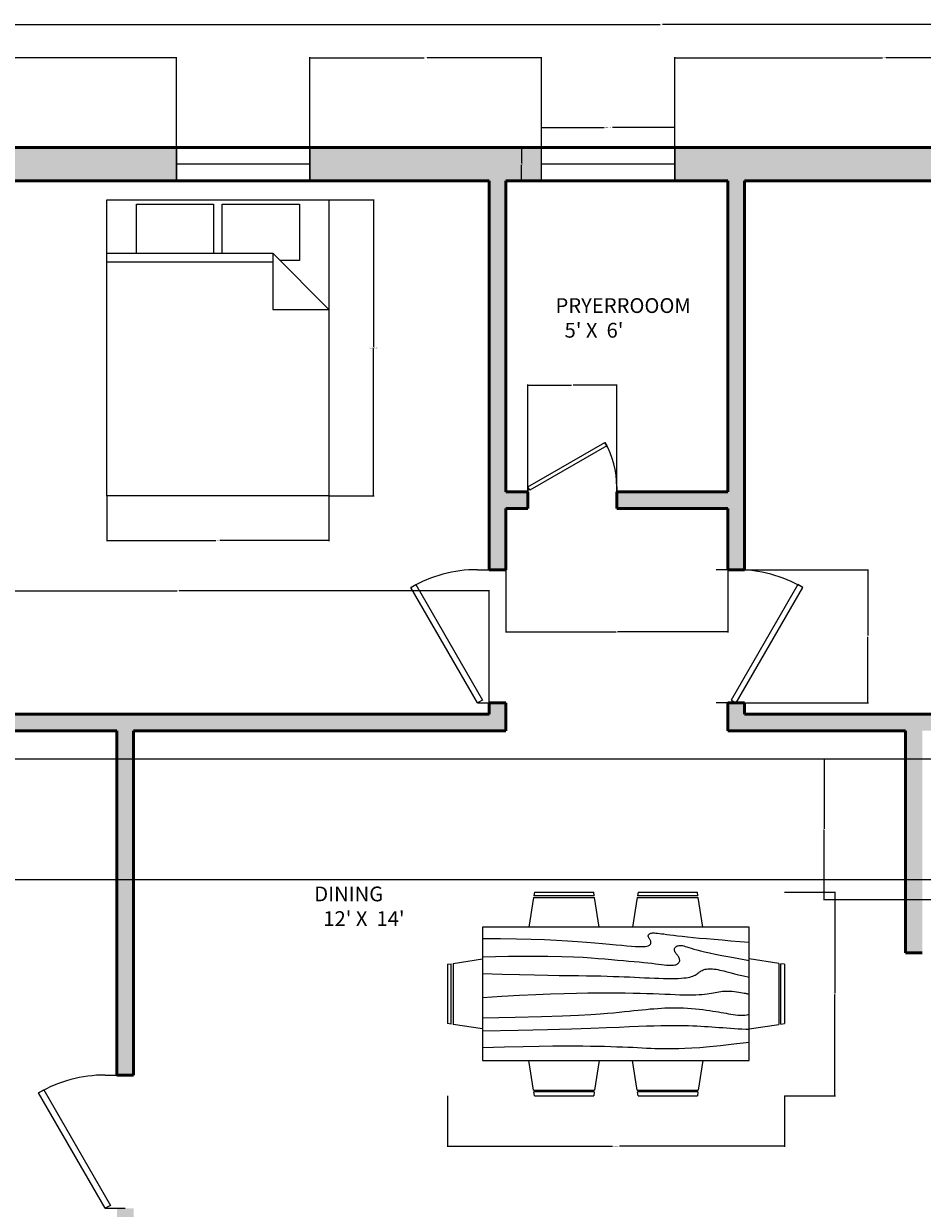
# Model space of a CAD drawing. Units: inches. Extents: x 4 to 671, y -79 to 570.
# Tile 4 of 7: x 165 to 408, y 250 to 570. Entities that reach past the tile are written whole.
import ezdxf

# ---------------------------------------------------------------- set-up
doc = ezdxf.new("R2010")
doc.units = ezdxf.units.IN
doc.header["$MEASUREMENT"] = 0
for name, color, linetype, lineweight in [('A-ANNO-DIMS', 2, 'Continuous', 18), ('A-AREA-IDEN', 7, 'Continuous', 18), ('A-WALL', 7, 'Continuous', 50), ('A-WALL-PATT', 251, 'Continuous', 13), ('doors', 40, 'Continuous', 25), ('furniture', 220, 'Continuous', 18), ('window', 30, 'Continuous', 25)]:
    doc.layers.add(name, color=color, linetype=linetype, lineweight=lineweight)
doc.styles.get("Standard").update_dxf_attribs({"font": 'arial.ttf'})
doc.dimstyles.get("Standard").update_dxf_attribs({"dimtxt": 0.18, "dimasz": 0.18, "dimexe": 0.18, "dimexo": 0.0625, "dimgap": 0.09, "dimtad": 0, "dimtih": 1, "dimtoh": 1, "dimdec": 4, "dimzin": 0, "dimdsep": 46, "dimtxsty": 'Standard', "dimcen": 0.09, "dimadec": 0, "dimazin": 0, "dimtfac": 1, "dimtdec": 4, "dimtofl": 0, "dimtmove": 0, "dimatfit": 3, "dimfxl": 1, "dimtolj": 1, "dimtzin": 0, "dimarcsym": 0})

# ---------------------------------------------------------------- blocks, each defined once
blk = doc.blocks.new('*U10')
for p, q in [((0, 0), (0, 6)), ((40, 0), (40, 6))]:
    blk.add_line(p, q)
blk.add_lwpolyline([(0, 0), (34.64, -20), (35.52, -18.48), (0.87, 1.52)], close=True)
blk.add_arc((0, 0), 40, 330, 0)
blk = doc.blocks.new('*U9')
for p, q in [((0, 0), (0, -6)), ((40, 0), (40, -6))]:
    blk.add_line(p, q)
blk.add_lwpolyline([(0, 0), (34.64, 20), (35.52, 18.48), (0.87, -1.52)], close=True)
blk.add_arc((0, 0), 40, 0, 30)
blk = doc.blocks.new('Bed - Queen')
for p, q in [((0, -80.00003), (0, 0)), ((0, 0), (59.99999, 0)), ((59.99999, 0), (59.99999, -80.00003)), ((7.99999, -1.2), (28.79998, -1.2)), ((7.99999, -14.4), (7.99999, -1.2)), ((28.79998, -1.2), (28.79998, -14.4)), ((31.19999, -1.2), (51.99999, -1.2)), ((31.19999, -14.4), (31.19999, -1.2)), ((51.99999, -1.2), (51.99999, -16.4)), ((0, -14.4), (44.8, -14.4)), ((59.99999, -29.6), (44.8, -14.4)), ((44.8, -14.4), (44.8, -29.6)), ((44.8, -16.8), (0, -16.8)), ((51.99999, -16.4), (46.79936, -16.4)), ((44.8, -29.6), (59.99999, -29.6)), ((59.99999, -80.00003), (0, -80.00003))]:
    blk.add_line(p, q)
blk = doc.blocks.new('Dining Set - 36 x 72 in.')
for p, q in [((-22.2343, 26.00059), (-23.4847, 17.99762)), ((-22.2304, 26), (-5.7608, 26)), ((-22, 27.5), (-22.1562, 26.50042)), ((-5.8416, 26.5), (-22.1534, 26.5)), ((-22, 27.5), (-6, 27.5)), ((-5.8437, 26.49966), (-6, 27.5)), ((-4.5152, 17.99762), (-5.7655, 25.99926)), ((5.7657, 26.00059), (4.5153, 17.99762)), ((5.7696, 26), (22.2392, 26)), ((6, 27.5), (5.8438, 26.50042)), ((22.1584, 26.5), (5.8466, 26.5)), ((6, 27.5), (22, 27.5)), ((22.1563, 26.49966), (22, 27.5)), ((23.4848, 17.99762), (22.2345, 25.99926)), ((36, 18), (-36, 18)), ((-36, 18), (-36, -18)), ((36, -18), (36, 18)), ((-45.5, 8), (-44.5004, 8.15617)), ((-45.5, 8), (-45.5, -8)), ((-44.5, -8.15843), (-44.5, 8.15338)), ((-44.0006, 8.23428), (-35.9976, 9.48474)), ((-44, 8.23041), (-44, -8.23915)), ((44.0006, 8.23428), (35.9976, 9.48474)), ((44, 8.23041), (44, -8.23915)), ((44.5, -8.15843), (44.5, 8.15338)), ((45.5, 8), (44.5005, 8.15617)), ((45.5, 8), (45.5, -8)), ((-44.4997, -8.15631), (-45.5, -8)), ((-35.9976, -9.48476), (-43.9993, -8.2345)), ((35.9976, -9.48476), (43.9993, -8.2345)), ((44.4997, -8.15631), (45.5, -8)), ((-36, -18), (36, -18)), ((-22.2343, -26.0006), (-23.4847, -17.99762)), ((-4.5152, -17.99762), (-5.7655, -25.99928)), ((5.7657, -26.0006), (4.5153, -17.99762)), ((23.4848, -17.99762), (22.2345, -25.99928)), ((-22.2304, -26), (-5.7608, -26)), ((-22, -27.5), (-22.1562, -26.50044)), ((-5.8416, -26.5), (-22.1534, -26.5)), ((-22, -27.5), (-6, -27.5)), ((-5.8437, -26.49967), (-6, -27.5)), ((5.7696, -26), (22.2392, -26)), ((6, -27.5), (5.8438, -26.50044)), ((22.1584, -26.5), (5.8466, -26.5)), ((6, -27.5), (22, -27.5)), ((22.1563, -26.49967), (22, -27.5))]:
    blk.add_line(p, q)
for points in [[(-36, 15), (-31.1772, 14.97754), (-26.8079, 14.91406), (-22.8538, 14.81543), (-19.276, 14.6875), (-16.0362, 14.53613), (-13.0957, 14.36718), (-10.4159, 14.18652), (-7.9583, 14), (-5.6904, 13.81315), (-3.6035, 13.63021), (-1.6954, 13.45508), (0.0365, 13.29166), (1.5945, 13.14388), (2.9811, 13.01562), (4.1988, 12.9108), (5.25, 12.83333), (6.1393, 12.78613), (6.8802, 12.76823), (7.4883, 12.77767), (7.9792, 12.8125), (8.3685, 12.87077), (8.6719, 12.95052), (8.9049, 13.0498), (9.0833, 13.16666), (9.2205, 13.29899), (9.3216, 13.44401), (9.3895, 13.59879), (9.4271, 13.76041), (9.4373, 13.92594), (9.4232, 14.09245), (9.3875, 14.257), (9.3333, 14.41666), (9.2638, 14.56917), (9.1836, 14.71484), (9.0975, 14.85465), (9.0104, 14.98958), (8.9272, 15.1206), (8.8529, 15.2487), (8.7922, 15.37483), (8.75, 15.5), (8.7305, 15.62467), (8.7344, 15.74739), (8.7617, 15.86621), (8.8125, 15.97916), (8.8867, 16.08431), (8.9844, 16.17968), (9.1055, 16.26334), (9.25, 16.33333), (9.4189, 16.38802), (9.6172, 16.42708), (9.8506, 16.45052), (10.125, 16.45833), (10.4463, 16.45052), (10.8203, 16.42708), (11.2529, 16.38802), (11.75, 16.33333), (12.3184, 16.26318), (12.9694, 16.17838), (13.7151, 16.07991), (14.5677, 15.96875), (15.5395, 15.84586), (16.6426, 15.71224), (17.8893, 15.56884), (19.2917, 15.41666), (20.859, 15.25667), (22.5879, 15.08984), (24.4721, 14.91715), (26.5052, 14.73958), (28.6809, 14.5581), (30.9929, 14.3737), (33.4347, 14.18733), (36, 14)], [(-36, 10), (-28.9766, 10.14274), (-23.1725, 10.20442), (-18.4241, 10.19775), (-14.5677, 10.13541), (-11.4399, 10.03011), (-8.877, 9.89453), (-6.7154, 9.74137), (-4.7917, 9.58333), (-2.9698, 9.43082), (-1.2246, 9.28515), (0.4415, 9.14534), (2.026, 9.01041), (3.5266, 8.87939), (4.9408, 8.7513), (6.266, 8.62516), (7.5, 8.5), (8.6411, 8.37549), (9.6914, 8.2539), (10.6538, 8.13818), (11.5312, 8.03125), (12.3267, 7.93603), (13.043, 7.85547), (13.6831, 7.79248), (14.25, 7.75), (14.7471, 7.7303), (15.1797, 7.73307), (15.5537, 7.75732), (15.875, 7.80208), (16.1494, 7.86637), (16.3828, 7.94922), (16.5811, 8.04964), (16.75, 8.16666), (16.8944, 8.29915), (17.0143, 8.44531), (17.1089, 8.60319), (17.1771, 8.77083), (17.218, 8.94629), (17.2305, 9.1276), (17.2137, 9.31282), (17.1667, 9.5), (17.0895, 9.6875), (16.987, 9.875), (16.8649, 10.0625), (16.7292, 10.25), (16.5856, 10.4375), (16.4401, 10.625), (16.2985, 10.8125), (16.1667, 11), (16.05, 11.18733), (15.9518, 11.3737), (15.8752, 11.5581), (15.8229, 11.73958), (15.798, 11.91715), (15.8034, 12.08984), (15.842, 12.25667), (15.9167, 12.41666), (16.0295, 12.56836), (16.1784, 12.70833), (16.3605, 12.83268), (16.5729, 12.9375), (16.8127, 13.01888), (17.0768, 13.07291), (17.3625, 13.0957), (17.6667, 13.08333), (17.9894, 13.03312), (18.3418, 12.94726), (18.7382, 12.82918), (19.1927, 12.68229), (19.7195, 12.51001), (20.3327, 12.31575), (21.0465, 12.10294), (21.875, 11.875), (22.8357, 11.63354), (23.959, 11.37304), (25.2786, 11.08618), (26.8282, 10.76562), (28.6414, 10.40405), (30.752, 9.99414), (33.1936, 9.52856), (36, 9)], [(-36, 5.5), (-30.7157, 5.3348), (-26.069, 5.20963), (-21.9946, 5.11767), (-18.4271, 5.05208), (-15.3009, 5.00602), (-12.5508, 4.97265), (-10.1112, 4.94515), (-7.9167, 4.91666), (-5.909, 4.88167), (-4.0586, 4.83984), (-2.3429, 4.79215), (-0.7396, 4.73958), (0.7739, 4.6831), (2.22, 4.6237), (3.6213, 4.56233), (5, 4.5), (6.373, 4.43782), (7.7344, 4.3776), (9.0723, 4.32129), (10.375, 4.27083), (11.6309, 4.22819), (12.8281, 4.19531), (13.9551, 4.17415), (15, 4.16666), (15.954, 4.17448), (16.819, 4.19791), (17.6001, 4.23698), (18.3021, 4.29166), (18.9299, 4.36198), (19.4883, 4.44791), (19.9823, 4.54948), (20.4167, 4.66666), (20.7969, 4.79899), (21.1302, 4.94401), (21.4245, 5.09879), (21.6875, 5.26041), (21.9271, 5.42594), (22.1511, 5.59245), (22.3672, 5.757), (22.5834, 5.91666), (22.8065, 6.06868), (23.0404, 6.21093), (23.2879, 6.34147), (23.5521, 6.45833), (23.8358, 6.55957), (24.142, 6.64323), (24.4735, 6.70735), (24.8334, 6.75), (25.2235, 6.76969), (25.642, 6.76692), (26.0858, 6.74267), (26.5521, 6.69791), (27.0379, 6.63362), (27.5404, 6.55078), (28.0565, 6.45036), (28.5834, 6.33333), (29.1242, 6.19987), (29.7071, 6.04687), (30.3661, 5.87044), (31.1354, 5.66666), (32.0493, 5.43164), (33.142, 5.16146), (34.4475, 4.85221), (36, 4.5)], [(-36, -1), (-30.7915, -0.6591), (-26.0195, -0.38216), (-21.6519, -0.16284), (-17.6563, 0.00521), (-14.0005, 0.12833), (-10.6523, 0.21289), (-7.5796, 0.26522), (-4.75, 0.29166), (-2.134, 0.29793), (0.2878, 0.28711), (2.5317, 0.26163), (4.6146, 0.22396), (6.5529, 0.17651), (8.3633, 0.12174), (10.0623, 0.06209), (11.6667, 0), (13.1899, -0.06201), (14.6341, -0.1211), (15.9982, -0.17432), (17.2813, -0.21875), (18.4823, -0.25147), (19.6003, -0.26953), (20.6343, -0.27002), (21.5834, -0.25), (22.4481, -0.20768), (23.2357, -0.14584), (23.9549, -0.06836), (24.6146, 0.02083), (25.2235, 0.11784), (25.7904, 0.21875), (26.3241, 0.31966), (26.8334, 0.41666), (27.3265, 0.50618), (27.8099, 0.58593), (28.2894, 0.65397), (28.7709, 0.70833), (29.2601, 0.74707), (29.763, 0.76823), (30.2855, 0.76985), (30.8334, 0.75), (31.4088, 0.70784), (31.9994, 0.64713), (32.589, 0.57275), (33.1615, 0.48958), (33.7008, 0.4025), (34.1908, 0.3164), (34.6153, 0.23616), (34.9584, 0.16666), (35.2099, 0.11165), (35.3848, 0.07031), (35.504, 0.04069), (35.5886, 0.02083), (35.6594, 0.00879), (35.7377, 0.0026), (35.8442, 0.00032), (36, 0)], [(-36, -6.5), (-27.1843, -6.31267), (-20.084, -6.1263), (-14.469, -5.9419), (-10.1094, -5.76042), (-6.7752, -5.58285), (-4.2363, -5.41016), (-2.2629, -5.24333), (-0.625, -5.08334), (0.8708, -4.93099), (2.2715, -4.78646), (3.5872, -4.64974), (4.8281, -4.52084), (6.0046, -4.39974), (7.127, -4.28646), (8.2053, -4.18099), (9.25, -4.08334), (10.2705, -3.99382), (11.2734, -3.91407), (12.2647, -3.84603), (13.25, -3.79167), (14.2354, -3.75293), (15.2266, -3.73177), (16.2295, -3.73015), (17.25, -3.75), (18.2912, -3.79248), (19.3451, -3.85547), (20.4009, -3.93604), (21.4479, -4.03125), (22.4754, -4.13819), (23.4727, -4.25391), (24.4289, -4.37549), (25.3334, -4.5), (26.1785, -4.62492), (26.9694, -4.74935), (27.7145, -4.87281), (28.4219, -4.99479), (29.1, -5.11483), (29.7572, -5.23242), (30.4016, -5.34709), (31.0417, -5.45834), (31.6837, -5.56437), (32.3262, -5.65821), (32.9658, -5.73153), (33.599, -5.77604), (34.2224, -5.78345), (34.8327, -5.74545), (35.4264, -5.65373), (36, -5.5)], [(-36, -10), (-26.4022, -9.81299), (-18.4675, -9.62891), (-11.9839, -9.45069), (-6.7396, -9.28125), (-2.5226, -9.12354), (0.8789, -8.98047), (3.6769, -8.85498), (6.0833, -8.75), (8.2767, -8.66765), (10.3021, -8.60677), (12.1712, -8.56543), (13.8958, -8.54167), (15.4876, -8.53353), (16.9583, -8.53907), (18.3197, -8.55632), (19.5834, -8.58334), (20.7616, -8.61841), (21.8685, -8.66081), (22.9188, -8.71004), (23.9271, -8.76563), (24.9081, -8.82707), (25.8763, -8.89388), (26.8465, -8.96558), (27.8334, -9.04167), (28.8474, -9.12118), (29.8828, -9.20117), (30.93, -9.27824), (31.9792, -9.34896), (33.0205, -9.40991), (34.0443, -9.45768), (35.0407, -9.48885), (36, -9.5)], [(-36, -14.5), (-30.0881, -14.33513), (-25.0332, -14.21224), (-20.7312, -14.12647), (-17.0781, -14.07292), (-13.97, -14.04671), (-11.3027, -14.04297), (-8.9724, -14.05681), (-6.875, -14.08334), (-4.9224, -14.11833), (-3.0905, -14.16016), (-1.3709, -14.20785), (0.2448, -14.26042), (1.7647, -14.3169), (3.1973, -14.3763), (4.5507, -14.43767), (5.8333, -14.5), (7.0554, -14.5621), (8.235, -14.62175), (9.3922, -14.67652), (10.5469, -14.72396), (11.7192, -14.76164), (12.929, -14.78711), (14.1965, -14.79794), (15.5417, -14.79167), (16.9933, -14.76424), (18.6152, -14.70508), (20.4804, -14.60197), (22.6615, -14.44271), (25.2312, -14.21509), (28.2624, -13.9069), (31.8277, -13.50594), (36, -13)]]:
    blk.add_lwpolyline(points)
blk = doc.blocks.new('WIN-36')
for p, q in [((0, 0), (0, 9)), ((0, 9), (36, 9)), ((36, 9), (36, 0)), ((36, 9), (36, 4.5)), ((36, 4.5), (0, 4.5)), ((36, 0), (0, 0))]:
    blk.add_line(p, q)
blk = doc.blocks.new('*D21')
at = {"layer": 'A-ANNO-DIMS', "color": 0, "lineweight": -2, "transparency": 16777216}
for p, q in [((305.11, 536.41), (305.11, 541.93)), ((305.29, 541.75), (321.99, 541.75)), ((340.93, 541.75), (324.23, 541.75)), ((341.11, 536.41), (341.11, 541.93))]:
    blk.add_line(p, q, dxfattribs=at)
at = {"layer": 'A-ANNO-DIMS', "color": 0, "transparency": 16777216}
for points in [[(305.29, 541.78), (305.29, 541.72), (305.11, 541.75)], [(340.93, 541.78), (340.93, 541.72), (341.11, 541.75)]]:
    blk.add_solid(points, dxfattribs=at)
at = {"layer": 'Defpoints', "color": 0, "transparency": 16777216}
for p in [(341.11, 541.75), (305.11, 536.35), (341.11, 536.35)]:
    blk.add_point(p, dxfattribs=at)
at = {"layer": 'A-ANNO-DIMS', "color": 0, "transparency": 16777216, "insert": (323.11, 541.75), "char_height": 0.18, "attachment_point": 5}
blk.add_mtext('\\A1;WINDOW 36 TYP.', dxfattribs=at)
blk = doc.blocks.new('*D22')
at = {"layer": 'A-ANNO-DIMS', "color": 0, "lineweight": -2, "transparency": 16777216}
for p, q in [((305.05, 536.35), (299.53, 536.35)), ((299.71, 536.17), (299.71, 532.03)), ((299.71, 527.53), (299.71, 531.67)), ((305.05, 527.35), (299.53, 527.35))]:
    blk.add_line(p, q, dxfattribs=at)
at = {"layer": 'A-ANNO-DIMS', "color": 0, "transparency": 16777216}
for points in [[(299.68, 536.17), (299.74, 536.17), (299.71, 536.35)], [(299.68, 527.53), (299.74, 527.53), (299.71, 527.35)]]:
    blk.add_solid(points, dxfattribs=at)
at = {"layer": 'Defpoints', "color": 0, "transparency": 16777216}
for p in [(299.71, 536.35), (305.11, 536.35), (305.11, 527.35)]:
    blk.add_point(p, dxfattribs=at)
at = {"layer": 'A-ANNO-DIMS', "color": 0, "transparency": 16777216, "insert": (299.71, 531.85), "char_height": 0.18, "attachment_point": 5}
blk.add_mtext('\\A1;9 TYP.', dxfattribs=at)
blk = doc.blocks.new('*D27')
at = {"layer": 'A-ANNO-DIMS', "color": 0, "lineweight": -2, "transparency": 16777216}
for p, q in [((247.76, 522.26), (259.87, 522.26)), ((259.69, 522.08), (259.69, 482.45)), ((259.69, 442.44), (259.69, 482.07)), ((247.76, 442.26), (259.87, 442.26))]:
    blk.add_line(p, q, dxfattribs=at)
at = {"layer": 'A-ANNO-DIMS', "color": 0, "transparency": 16777216}
for points in [[(259.66, 522.08), (259.72, 522.08), (259.69, 522.26)], [(259.66, 442.44), (259.72, 442.44), (259.69, 442.26)]]:
    blk.add_solid(points, dxfattribs=at)
at = {"layer": 'Defpoints', "color": 0, "transparency": 16777216}
for p in [(247.69, 522.26), (259.69, 522.26), (247.69, 442.26)]:
    blk.add_point(p, dxfattribs=at)
at = {"layer": 'A-ANNO-DIMS', "color": 0, "transparency": 16777216, "insert": (259.69, 482.26), "char_height": 0.18, "attachment_point": 5}
blk.add_mtext('\\A1;QUEEN BED 80 TYP.', dxfattribs=at)
blk = doc.blocks.new('*D28')
at = {"layer": 'A-ANNO-DIMS', "color": 0, "lineweight": -2, "transparency": 16777216}
for p, q in [((187.69, 442.2), (187.69, 430.08)), ((247.69, 442.2), (247.69, 430.08)), ((187.87, 430.26), (217.17, 430.26)), ((247.51, 430.26), (218.22, 430.26))]:
    blk.add_line(p, q, dxfattribs=at)
at = {"layer": 'A-ANNO-DIMS', "color": 0, "transparency": 16777216}
for points in [[(187.87, 430.29), (187.87, 430.23), (187.69, 430.26)], [(247.51, 430.29), (247.51, 430.23), (247.69, 430.26)]]:
    blk.add_solid(points, dxfattribs=at)
at = {"layer": 'Defpoints', "color": 0, "transparency": 16777216}
for p in [(187.69, 442.26), (247.69, 442.26), (247.69, 430.26)]:
    blk.add_point(p, dxfattribs=at)
at = {"layer": 'A-ANNO-DIMS', "color": 0, "transparency": 16777216, "insert": (217.69, 430.26), "char_height": 0.18, "attachment_point": 5}
blk.add_mtext('\\A1;60 TYP.', dxfattribs=at)
blk = doc.blocks.new('*D41')
at = {"layer": 'A-ANNO-DIMS', "color": 0, "lineweight": -2, "transparency": 16777216}
for p, q in [((279.69, 280.21), (279.69, 266.44)), ((370.69, 280.21), (370.69, 266.44)), ((279.87, 266.62), (324.24, 266.62)), ((370.51, 266.62), (326.15, 266.62))]:
    blk.add_line(p, q, dxfattribs=at)
at = {"layer": 'A-ANNO-DIMS', "color": 0, "transparency": 16777216}
for points in [[(279.87, 266.65), (279.87, 266.59), (279.69, 266.62)], [(370.51, 266.65), (370.51, 266.59), (370.69, 266.62)]]:
    blk.add_solid(points, dxfattribs=at)
at = {"layer": 'Defpoints', "color": 0, "transparency": 16777216}
for p in [(279.69, 280.27), (370.69, 280.27), (370.69, 266.62)]:
    blk.add_point(p, dxfattribs=at)
at = {"layer": 'A-ANNO-DIMS', "color": 0, "transparency": 16777216, "insert": (325.19, 266.62), "char_height": 0.18, "attachment_point": 5}
blk.add_mtext('\\A1;DINING SET 91', dxfattribs=at)
blk = doc.blocks.new('*D42')
at = {"layer": 'A-ANNO-DIMS', "color": 0, "lineweight": -2, "transparency": 16777216}
for p, q in [((370.76, 335.27), (384.52, 335.27)), ((384.34, 335.09), (384.34, 307.95)), ((384.34, 280.45), (384.34, 307.59)), ((370.76, 280.27), (384.52, 280.27))]:
    blk.add_line(p, q, dxfattribs=at)
at = {"layer": 'A-ANNO-DIMS', "color": 0, "transparency": 16777216}
for points in [[(384.31, 335.09), (384.37, 335.09), (384.34, 335.27)], [(384.31, 280.45), (384.37, 280.45), (384.34, 280.27)]]:
    blk.add_solid(points, dxfattribs=at)
at = {"layer": 'Defpoints', "color": 0, "transparency": 16777216}
for p in [(370.69, 335.27), (384.34, 335.27), (370.69, 280.27)]:
    blk.add_point(p, dxfattribs=at)
at = {"layer": 'A-ANNO-DIMS', "color": 0, "transparency": 16777216, "insert": (384.34, 307.77), "char_height": 0.18, "attachment_point": 5}
blk.add_mtext('\\A1;55', dxfattribs=at)
blk = doc.blocks.new('*D49')
at = {"layer": 'A-ANNO-DIMS', "color": 0, "lineweight": -2, "transparency": 16777216}
for p, q in [((37.44, 536.41), (37.44, 569.83)), ((37.62, 569.65), (337.15, 569.65)), ((637.26, 569.65), (337.73, 569.65)), ((637.44, 536.41), (637.44, 569.83))]:
    blk.add_line(p, q, dxfattribs=at)
at = {"layer": 'A-ANNO-DIMS', "color": 0, "transparency": 16777216}
for points in [[(37.62, 569.68), (37.62, 569.62), (37.44, 569.65)], [(637.26, 569.68), (637.26, 569.62), (637.44, 569.65)]]:
    blk.add_solid(points, dxfattribs=at)
at = {"layer": 'Defpoints', "color": 0, "transparency": 16777216}
for p in [(637.44, 569.65), (37.44, 536.35), (637.44, 536.35)]:
    blk.add_point(p, dxfattribs=at)
at = {"layer": 'A-ANNO-DIMS', "color": 0, "transparency": 16777216, "insert": (337.44, 569.65), "char_height": 0.18, "attachment_point": 5}
blk.add_mtext('\\A1;600', dxfattribs=at)
blk = doc.blocks.new('*D50')
at = {"layer": 'A-ANNO-DIMS', "color": 0, "lineweight": -2, "transparency": 16777216}
for p, q in [((637.5, 536.35), (670.92, 536.35)), ((670.74, 536.17), (670.74, 245.53)), ((670.74, -45.47), (670.74, 245.17)), ((389.27, -45.65), (670.92, -45.65))]:
    blk.add_line(p, q, dxfattribs=at)
at = {"layer": 'A-ANNO-DIMS', "color": 0, "transparency": 16777216}
for points in [[(670.71, 536.17), (670.77, 536.17), (670.74, 536.35)], [(670.71, -45.47), (670.77, -45.47), (670.74, -45.65)]]:
    blk.add_solid(points, dxfattribs=at)
at = {"layer": 'Defpoints', "color": 0, "transparency": 16777216}
for p in [(637.44, 536.35), (389.21, -45.65), (670.74, -45.65)]:
    blk.add_point(p, dxfattribs=at)
at = {"layer": 'A-ANNO-DIMS', "color": 0, "transparency": 16777216, "insert": (670.74, 245.35), "char_height": 0.18, "attachment_point": 5}
blk.add_mtext('\\A1;582', dxfattribs=at)
blk = doc.blocks.new('*D59')
at = {"layer": 'A-ANNO-DIMS', "color": 0, "lineweight": -2, "transparency": 16777216}
for p, q in [((122.94, 383.41), (122.94, 416.83)), ((123.12, 416.65), (206.66, 416.65)), ((290.76, 416.65), (207.22, 416.65)), ((290.94, 383.41), (290.94, 416.83))]:
    blk.add_line(p, q, dxfattribs=at)
at = {"layer": 'A-ANNO-DIMS', "color": 0, "transparency": 16777216}
for points in [[(123.12, 416.68), (123.12, 416.62), (122.94, 416.65)], [(290.76, 416.68), (290.76, 416.62), (290.94, 416.65)]]:
    blk.add_solid(points, dxfattribs=at)
at = {"layer": 'Defpoints', "color": 0, "transparency": 16777216}
for p in [(290.94, 416.65), (122.94, 383.35), (290.94, 383.35)]:
    blk.add_point(p, dxfattribs=at)
at = {"layer": 'A-ANNO-DIMS', "color": 0, "transparency": 16777216, "insert": (206.94, 416.65), "char_height": 0.18, "attachment_point": 5}
blk.add_mtext('\\A1;168', dxfattribs=at)
blk = doc.blocks.new('*D62')
at = {"layer": 'A-ANNO-DIMS', "color": 0, "lineweight": -2, "transparency": 16777216}
for p, q in [((301.44, 438.91), (301.44, 472.33)), ((301.62, 472.15), (313.22, 472.15)), ((325.26, 472.15), (313.66, 472.15)), ((325.44, 438.91), (325.44, 472.33))]:
    blk.add_line(p, q, dxfattribs=at)
at = {"layer": 'A-ANNO-DIMS', "color": 0, "transparency": 16777216}
for points in [[(301.62, 472.18), (301.62, 472.12), (301.44, 472.15)], [(325.26, 472.18), (325.26, 472.12), (325.44, 472.15)]]:
    blk.add_solid(points, dxfattribs=at)
at = {"layer": 'Defpoints', "color": 0, "transparency": 16777216}
for p in [(325.44, 472.15), (301.44, 438.85), (325.44, 438.85)]:
    blk.add_point(p, dxfattribs=at)
at = {"layer": 'A-ANNO-DIMS', "color": 0, "transparency": 16777216, "insert": (313.44, 472.15), "char_height": 0.18, "attachment_point": 5}
blk.add_mtext('\\A1;24', dxfattribs=at)
blk = doc.blocks.new('*D81')
at = {"layer": 'A-ANNO-DIMS', "color": 0, "lineweight": -2, "transparency": 16777216}
for p, q in [((93.01, 527.41), (93.01, 560.83)), ((93.19, 560.65), (149.33, 560.65)), ((206.38, 560.65), (150.24, 560.65)), ((206.56, 527.41), (206.56, 560.83))]:
    blk.add_line(p, q, dxfattribs=at)
at = {"layer": 'A-ANNO-DIMS', "color": 0, "transparency": 16777216}
for points in [[(93.19, 560.68), (93.19, 560.62), (93.01, 560.65)], [(206.38, 560.68), (206.38, 560.62), (206.56, 560.65)]]:
    blk.add_solid(points, dxfattribs=at)
at = {"layer": 'Defpoints', "color": 0, "transparency": 16777216}
for p in [(206.56, 560.65), (93.01, 527.35), (206.56, 527.35)]:
    blk.add_point(p, dxfattribs=at)
at = {"layer": 'A-ANNO-DIMS', "color": 0, "transparency": 16777216, "insert": (149.79, 560.65), "char_height": 0.18, "attachment_point": 5}
blk.add_mtext('\\A1;113.55', dxfattribs=at)
blk = doc.blocks.new('*D82')
at = {"layer": 'A-ANNO-DIMS', "color": 0, "lineweight": -2, "transparency": 16777216}
for p, q in [((242.56, 527.41), (242.56, 560.83)), ((242.74, 560.65), (273.44, 560.65)), ((304.93, 560.65), (274.23, 560.65)), ((305.11, 527.41), (305.11, 560.83))]:
    blk.add_line(p, q, dxfattribs=at)
at = {"layer": 'A-ANNO-DIMS', "color": 0, "transparency": 16777216}
for points in [[(242.74, 560.68), (242.74, 560.62), (242.56, 560.65)], [(304.93, 560.68), (304.93, 560.62), (305.11, 560.65)]]:
    blk.add_solid(points, dxfattribs=at)
at = {"layer": 'Defpoints', "color": 0, "transparency": 16777216}
for p in [(305.11, 560.65), (242.56, 527.35), (305.11, 527.35)]:
    blk.add_point(p, dxfattribs=at)
at = {"layer": 'A-ANNO-DIMS', "color": 0, "transparency": 16777216, "insert": (273.84, 560.65), "char_height": 0.18, "attachment_point": 5}
blk.add_mtext('\\A1;62.55', dxfattribs=at)
blk = doc.blocks.new('*D83')
at = {"layer": 'A-ANNO-DIMS', "color": 0, "lineweight": -2, "transparency": 16777216}
for p, q in [((341.11, 527.41), (341.11, 560.83)), ((341.29, 560.65), (397.17, 560.65)), ((453.95, 560.65), (398.07, 560.65)), ((454.13, 527.41), (454.13, 560.83))]:
    blk.add_line(p, q, dxfattribs=at)
at = {"layer": 'A-ANNO-DIMS', "color": 0, "transparency": 16777216}
for points in [[(341.29, 560.68), (341.29, 560.62), (341.11, 560.65)], [(453.95, 560.68), (453.95, 560.62), (454.13, 560.65)]]:
    blk.add_solid(points, dxfattribs=at)
at = {"layer": 'Defpoints', "color": 0, "transparency": 16777216}
for p in [(454.13, 560.65), (341.11, 527.35), (454.13, 527.35)]:
    blk.add_point(p, dxfattribs=at)
at = {"layer": 'A-ANNO-DIMS', "color": 0, "transparency": 16777216, "insert": (397.62, 560.65), "char_height": 0.18, "attachment_point": 5}
blk.add_mtext('\\A1;113.02', dxfattribs=at)
blk = doc.blocks.new('*D91')
at = {"layer": 'A-ANNO-DIMS', "color": 0, "lineweight": -2, "transparency": 16777216}
for p, q in [((414.71, 371.2), (381.29, 371.2)), ((381.47, 371.02), (381.47, 352.37)), ((381.47, 333.35), (381.47, 352)), ((414.71, 333.17), (381.29, 333.17))]:
    blk.add_line(p, q, dxfattribs=at)
at = {"layer": 'A-ANNO-DIMS', "color": 0, "transparency": 16777216}
for points in [[(381.44, 371.02), (381.5, 371.02), (381.47, 371.2)], [(381.44, 333.35), (381.5, 333.35), (381.47, 333.17)]]:
    blk.add_solid(points, dxfattribs=at)
at = {"layer": 'Defpoints', "color": 0, "transparency": 16777216}
for p in [(381.47, 371.2), (414.77, 371.2), (414.77, 333.17)]:
    blk.add_point(p, dxfattribs=at)
at = {"layer": 'A-ANNO-DIMS', "color": 0, "transparency": 16777216, "insert": (381.47, 352.18), "char_height": 0.18, "attachment_point": 5}
blk.add_mtext('\\A1;38.04', dxfattribs=at)
blk = doc.blocks.new('*D94')
at = {"layer": 'A-ANNO-DIMS', "color": 0, "lineweight": -2, "transparency": 16777216}
for p, q in [((515.23, 371.2), (3.96, 371.2)), ((4.14, 371.02), (4.14, 355.08)), ((4.14, 338.78), (4.14, 354.72)), ((515.23, 338.6), (3.96, 338.6))]:
    blk.add_line(p, q, dxfattribs=at)
at = {"layer": 'A-ANNO-DIMS', "color": 0, "transparency": 16777216}
for points in [[(4.11, 371.02), (4.17, 371.02), (4.14, 371.2)], [(4.11, 338.78), (4.17, 338.78), (4.14, 338.6)]]:
    blk.add_solid(points, dxfattribs=at)
at = {"layer": 'Defpoints', "color": 0, "transparency": 16777216}
for p in [(4.14, 371.2), (515.3, 371.2), (515.3, 338.6)]:
    blk.add_point(p, dxfattribs=at)
at = {"layer": 'A-ANNO-DIMS', "color": 0, "transparency": 16777216, "insert": (4.14, 354.9), "char_height": 0.18, "attachment_point": 5}
blk.add_mtext('\\A1;32.6', dxfattribs=at)
blk = doc.blocks.new('*D98')
at = {"layer": 'A-ANNO-DIMS', "color": 0, "lineweight": -2, "transparency": 16777216}
for p, q in [((295.44, 438.79), (295.44, 405.37)), ((355.44, 438.79), (355.44, 405.37)), ((295.62, 405.55), (325.22, 405.55)), ((355.26, 405.55), (325.66, 405.55))]:
    blk.add_line(p, q, dxfattribs=at)
at = {"layer": 'A-ANNO-DIMS', "color": 0, "transparency": 16777216}
for points in [[(295.62, 405.58), (295.62, 405.52), (295.44, 405.55)], [(355.26, 405.58), (355.26, 405.52), (355.44, 405.55)]]:
    blk.add_solid(points, dxfattribs=at)
at = {"layer": 'Defpoints', "color": 0, "transparency": 16777216}
for p in [(295.44, 438.85), (355.44, 438.85), (295.44, 405.55)]:
    blk.add_point(p, dxfattribs=at)
at = {"layer": 'A-ANNO-DIMS', "color": 0, "transparency": 16777216, "insert": (325.44, 405.55), "char_height": 0.18, "attachment_point": 5}
blk.add_mtext('\\A1;60', dxfattribs=at)
blk = doc.blocks.new('*D99')
at = {"layer": 'A-ANNO-DIMS', "color": 0, "lineweight": -2, "transparency": 16777216}
for p, q in [((360, 422.35), (393.42, 422.35)), ((393.24, 422.17), (393.24, 404.53)), ((393.24, 386.53), (393.24, 404.17)), ((360, 386.35), (393.42, 386.35))]:
    blk.add_line(p, q, dxfattribs=at)
at = {"layer": 'A-ANNO-DIMS', "color": 0, "transparency": 16777216}
for points in [[(393.21, 422.17), (393.27, 422.17), (393.24, 422.35)], [(393.21, 386.53), (393.27, 386.53), (393.24, 386.35)]]:
    blk.add_solid(points, dxfattribs=at)
at = {"layer": 'Defpoints', "color": 0, "transparency": 16777216}
for p in [(359.94, 422.35), (359.94, 386.35), (393.24, 386.35)]:
    blk.add_point(p, dxfattribs=at)
at = {"layer": 'A-ANNO-DIMS', "color": 0, "transparency": 16777216, "insert": (393.24, 404.35), "char_height": 0.18, "attachment_point": 5}
blk.add_mtext('\\A1;36', dxfattribs=at)

msp = doc.modelspace()

# ---------------------------------------------------------------- hatches: boundary and pattern name
at = {"layer": 'A-WALL-PATT'}
h = msp.add_hatch(color=256, dxfattribs=at)
h.dxf.hatch_style = 1
h.paths.add_polyline_path([(46.4392, 165.2664), (37.4392, 165.2664), (37.4392, 108.5522), (41.9392, 108.5522), (46.4392, 108.5522), (46.4392, 117.8513), (151.434, 117.8513), (151.434, 120.1013), (151.434, 122.3513), (46.4392, 122.3513)], flags=17)
h.paths.add_polyline_path([(194.9392, 203.3513), (190.4392, 203.3513), (190.4392, 122.3513), (187.434, 122.3513), (187.434, 117.8513), (190.4392, 117.8513), (190.4392, 65.3513), (46.4392, 65.3513), (46.4392, 72.5522), (37.4392, 72.5522), (37.4392, 56.3513), (218.8007, 56.3513), (218.8007, 65.3513), (194.9392, 65.3513)])
h.paths.add_polyline_path([(46.4392, 242.3513), (190.4392, 242.3513), (190.4392, 239.3513), (194.9392, 239.3513), (194.9392, 249.8513), (190.4392, 249.8513), (190.4392, 246.8513), (46.4392, 246.8513), (46.4392, 303.5372), (37.4392, 303.5372), (37.4392, 201.2664), (41.9392, 201.2664), (46.4392, 201.2664)])
h.paths.add_polyline_path([(46.4392, 378.8513), (190.4392, 378.8513), (190.4392, 285.8513), (194.9392, 285.8513), (194.9392, 378.8513), (295.4392, 378.8513), (295.4392, 386.3513), (290.9392, 386.3513), (290.9392, 383.3513), (122.9392, 383.3513), (122.9392, 386.3513), (118.4392, 386.3513), (118.4392, 383.3513), (46.4392, 383.3513), (46.4392, 438.8513), (79.4392, 438.8513), (79.4392, 443.3513), (46.4392, 443.3513), (46.4392, 527.3513), (57.0095, 527.3513), (57.0095, 536.3513), (37.4392, 536.3513), (37.4392, 339.5372), (41.9392, 339.5372), (46.4392, 339.5372)])
h = msp.add_hatch(color=256, dxfattribs=at)
h.dxf.hatch_style = 1
h.paths.add_polyline_path([(206.5642, 536.3513), (93.0095, 536.3513), (93.0095, 531.8513), (93.0095, 527.3513), (118.4392, 527.3513), (118.4392, 443.3513), (115.4392, 443.3513), (115.4392, 438.8513), (118.4392, 438.8513), (118.4392, 422.3513), (120.6892, 422.3513), (122.9392, 422.3513), (122.9392, 527.3513), (206.5642, 527.3513)])
h.paths.add_polyline_path([(305.1113, 536.3513), (242.5642, 536.3513), (242.5642, 531.8513), (242.5642, 527.3513), (290.9392, 527.3513), (290.9392, 422.3513), (293.1892, 422.3513), (295.4392, 422.3513), (295.4392, 438.8513), (301.4392, 438.8513), (301.4392, 443.3513), (295.4392, 443.3513), (295.4392, 527.3513), (305.1113, 527.3513)])
h.paths.add_polyline_path([(454.1293, 536.3513), (341.1113, 536.3513), (341.1113, 531.8513), (341.1113, 527.3513), (355.4392, 527.3513), (355.4392, 443.3513), (325.4392, 443.3513), (325.4392, 438.8513), (355.4392, 438.8513), (355.4392, 422.3513), (359.9392, 422.3513), (359.9392, 527.3513), (454.1293, 527.3513)])
h.paths.add_polyline_path([(637.4392, 536.3513), (490.1293, 536.3513), (490.1293, 531.8513), (490.1293, 527.3513), (527.9392, 527.3513), (527.9392, 505.9443), (532.4392, 505.9443), (532.4392, 527.3513), (628.4392, 527.3513), (628.4392, 500.2662), (637.4392, 500.2662)])
h.paths.add_polyline_path([(637.4392, 464.2662), (628.4392, 464.2662), (628.4392, 383.3513), (556.4392, 383.3513), (532.4392, 383.3513), (532.4392, 469.9443), (527.9392, 469.9443), (527.9392, 383.3513), (359.9392, 383.3513), (359.9392, 386.3513), (355.4392, 386.3513), (355.4392, 378.8513), (403.4392, 378.8513), (403.4392, 318.8513), (407.9392, 318.8513), (407.9392, 378.8513), (551.9392, 378.8513), (551.9392, 290.3513), (554.1892, 290.3513, -0.01563646), (556.4392, 290.2809), (556.4392, 378.8513), (628.4392, 378.8513), (628.4392, 342.8513), (637.4392, 342.8513)])

# ---------------------------------------------------------------- linework, layer by layer
at = {"layer": 'A-WALL'}
for p, q in [((122.9392, 527.3513), (290.9392, 527.3513)), ((290.9392, 422.3513), (290.9392, 527.3513)), ((295.4392, 527.3513), (355.4392, 527.3513)), ((295.4392, 443.3513), (295.4392, 527.3513)), ((355.4392, 443.3513), (355.4392, 527.3513)), ((359.9392, 527.3513), (527.9392, 527.3513)), ((359.9392, 422.3513), (359.9392, 527.3513)), ((295.4392, 443.3513), (301.4392, 443.3513)), ((301.4392, 443.3513), (301.4392, 438.8513)), ((325.4392, 443.3513), (355.4392, 443.3513)), ((325.4392, 438.8513), (325.4392, 443.3513)), ((295.4392, 438.8513), (301.4392, 438.8513)), ((295.4392, 422.3513), (295.4392, 438.8513)), ((325.4392, 438.8513), (355.4392, 438.8513)), ((355.4392, 422.3513), (355.4392, 438.8513)), ((290.9392, 422.3513), (295.4392, 422.3513)), ((355.4392, 422.3513), (359.9392, 422.3513)), ((290.9392, 386.3513), (295.4392, 386.3513)), ((290.9392, 383.3513), (290.9392, 386.3513)), ((295.4392, 378.8513), (295.4392, 386.3513)), ((355.4392, 386.3513), (359.9392, 386.3513)), ((355.4392, 378.8513), (355.4392, 386.3513)), ((359.9392, 383.3513), (359.9392, 386.3513)), ((122.9392, 383.3513), (290.9392, 383.3513)), ((122.9392, 383.3513), (290.9392, 383.3513)), ((359.9392, 383.3513), (527.9392, 383.3513)), ((46.4392, 378.8513), (190.4392, 378.8513)), ((46.4392, 378.8513), (190.4392, 378.8513)), ((190.4392, 285.8513), (190.4392, 378.8513)), ((194.9392, 378.8513), (295.4392, 378.8513)), ((194.9392, 378.8513), (295.4392, 378.8513)), ((194.9392, 285.8513), (194.9392, 378.8513)), ((355.4392, 378.8513), (403.4392, 378.8513)), ((403.4392, 378.8513), (403.4392, 318.8513)), ((403.4392, 318.8513), (407.9392, 318.8513)), ((190.4392, 285.8513), (194.9392, 285.8513))]:
    msp.add_line(p, q, dxfattribs=at)
msp.add_lwpolyline([(313.4392, 56.3513), (37.4392, 56.3513), (37.4392, 536.3513), (637.4392, 536.3513), (637.4392, 56.3513), (362.9392, 56.3513)], dxfattribs=at)

# ---------------------------------------------------------------- block references
at = {"layer": 'doors', "xscale": 0.5999999999999549, "yscale": 0.5999999999999549, "zscale": 0.5999999999999549}
msp.add_blockref('*U9', (301.4392, 444.7013), dxfattribs=at)
at = {"layer": 'doors', "xscale": 0.9, "yscale": 0.9, "zscale": 0.9}
for name, p, rotation in [('*U9', (287.7892, 386.3513), 89.99999999995367), ('*U10', (357.6892, 386.3513), 90), ('*U9', (187.2892, 249.8513), 89.99999999995367)]:
    msp.add_blockref(name, p, dxfattribs=dict(at, rotation=rotation))
at = {"layer": 'furniture'}
for name, p in [('Bed - Queen', (187.694, 522.2606)), ('Dining Set - 36 x 72 in.', (325.1949, 307.7705))]:
    msp.add_blockref(name, p, dxfattribs=at)
at = {"layer": 'window'}
for p in [(206.5638, 527.351), (305.111, 527.351)]:
    msp.add_blockref('WIN-36', p, dxfattribs=at)

# ---------------------------------------------------------------- texts
at = {"layer": 'A-AREA-IDEN', "char_height": 4, "attachment_point": 1}
for s, insert in [("PRYERROOOM\\P  5' X  6'", (308.881, 495.6921)), ("DINING\\P  12' X  14'", (243.7236, 336.771))]:
    msp.add_mtext_dynamic_manual_height_columns(s, width=44.806469, gutter_width=1, heights=[0], dxfattribs=dict(at, insert=insert))

# ---------------------------------------------------------------- dimensions: what is measured, and where the dimension line sits
at = {"layer": 'A-ANNO-DIMS'}
for base, p1, p2, override, picture, middle in [((637.4392, 569.6513), (37.4392, 536.3513), (637.4392, 536.3513), {"dimdec": 0, "dimlfac": 1, "dimrnd": 0, "dimzin": 0, "dimdsep": 46, "dimlunit": 2}, '*D49', (337.4392, 569.6513)), ((206.5642, 560.6513), (93.0095, 527.3513), (206.5642, 527.3513), {"dimdec": 2, "dimlfac": 1, "dimrnd": 0, "dimzin": 0, "dimdsep": 46, "dimlunit": 2}, '*D81', (149.7868, 560.6513)), ((305.1113, 560.6513), (242.5642, 527.3513), (305.1113, 527.3513), {"dimdec": 2, "dimlfac": 1, "dimrnd": 0, "dimzin": 0, "dimdsep": 46, "dimlunit": 2}, '*D82', (273.8378, 560.6513)), ((454.1293, 560.6513), (341.1113, 527.3513), (454.1293, 527.3513), {"dimdec": 2, "dimlfac": 1, "dimrnd": 0, "dimzin": 0, "dimdsep": 46, "dimlunit": 2}, '*D83', (397.6203, 560.6513)), ((325.4392, 472.1513), (301.4392, 438.8513), (325.4392, 438.8513), {"dimdec": 0, "dimlfac": 1, "dimrnd": 0, "dimzin": 0, "dimdsep": 46, "dimlunit": 2}, '*D62', (313.4392, 472.1513)), ((290.9392, 416.6513), (122.9392, 383.3513), (290.9392, 383.3513), {"dimdec": 0, "dimlfac": 1, "dimrnd": 0, "dimzin": 0, "dimdsep": 46, "dimlunit": 2}, '*D59', (206.9392, 416.6513))]:
    dim = msp.add_linear_dim(base=base, p1=p1, p2=p2, dimstyle='Standard', override=override, dxfattribs=at)
    dim.commit()
    dim.dimension.update_dxf_attribs({"geometry": picture, "text_midpoint": middle})
for base, p1, p2, text, picture, middle in [((341.1113, 541.7513), (305.1113, 536.3513), (341.1113, 536.3513), 'WINDOW <> TYP.', '*D21', (323.1113, 541.7513)), ((247.694, 430.2606), (187.694, 442.2606), (247.694, 442.2606), '<> TYP.', '*D28', (217.694, 430.2606)), ((370.6949, 266.6205), (279.6949, 280.2705), (370.6949, 280.2705), 'DINING SET <>', '*D41', (325.1949, 266.6205))]:
    dim = msp.add_linear_dim(base=base, p1=p1, p2=p2, text=text, dimstyle='Standard', override={"dimdec": 0, "dimlfac": 1, "dimrnd": 0, "dimzin": 0, "dimdsep": 46, "dimlunit": 2}, dxfattribs=at)
    dim.commit()
    dim.dimension.update_dxf_attribs({"geometry": picture, "text_midpoint": middle})
for base, p1, p2, text, picture, middle in [((299.7113, 536.3513), (305.1113, 527.3513), (305.1113, 536.3513), '<> TYP.', '*D22', (299.7113, 531.8513)), ((259.694, 522.2606), (247.694, 442.2606), (247.694, 522.2606), 'QUEEN BED <> TYP.', '*D27', (259.694, 482.2606))]:
    dim = msp.add_linear_dim(base=base, p1=p1, p2=p2, angle=90, text=text, dimstyle='Standard', override={"dimdec": 0, "dimlfac": 1, "dimrnd": 0, "dimzin": 0, "dimdsep": 46, "dimlunit": 2}, dxfattribs=at)
    dim.commit()
    dim.dimension.update_dxf_attribs({"geometry": picture, "text_midpoint": middle})
for base, p1, p2, angle, override, picture, middle in [((670.7392, -45.6487), (637.4392, 536.3513), (389.2077, -45.6487), 90, {"dimdec": 0, "dimlfac": 1, "dimrnd": 0, "dimzin": 0, "dimdsep": 46, "dimlunit": 2}, '*D50', (670.7392, 245.3513)), ((295.4392, 405.5513), (355.4392, 438.8513), (295.4392, 438.8513), 180, {"dimdec": 0, "dimlfac": 1, "dimrnd": 0, "dimzin": 0, "dimdsep": 46, "dimlunit": 2}, '*D98', (325.4392, 405.5513)), ((393.2392, 386.3513), (359.9392, 422.3513), (359.9392, 386.3513), 270, {"dimdec": 0, "dimlfac": 1, "dimrnd": 0, "dimzin": 0, "dimdsep": 46, "dimlunit": 2}, '*D99', (393.2392, 404.3513)), ((4.1392, 371.2019), (515.2973, 338.599), (515.2973, 371.2019), 90, {"dimdec": 1, "dimlfac": 1, "dimrnd": 0, "dimzin": 0, "dimdsep": 46, "dimlunit": 2}, '*D94', (4.1392, 354.9005)), ((381.4716, 371.2019), (414.7716, 333.1651), (414.7716, 371.2019), 90, {"dimdec": 2, "dimlfac": 1, "dimrnd": 0, "dimzin": 0, "dimdsep": 46, "dimlunit": 2}, '*D91', (381.4716, 352.1835)), ((384.3449, 335.2705), (370.6949, 280.2705), (370.6949, 335.2705), 90, {"dimdec": 0, "dimlfac": 1, "dimrnd": 0, "dimzin": 0, "dimdsep": 46, "dimlunit": 2}, '*D42', (384.3449, 307.7705))]:
    dim = msp.add_linear_dim(base=base, p1=p1, p2=p2, angle=angle, dimstyle='Standard', override=override, dxfattribs=at)
    dim.commit()
    dim.dimension.update_dxf_attribs({"geometry": picture, "text_midpoint": middle})

doc.saveas('drawing.dxf')
